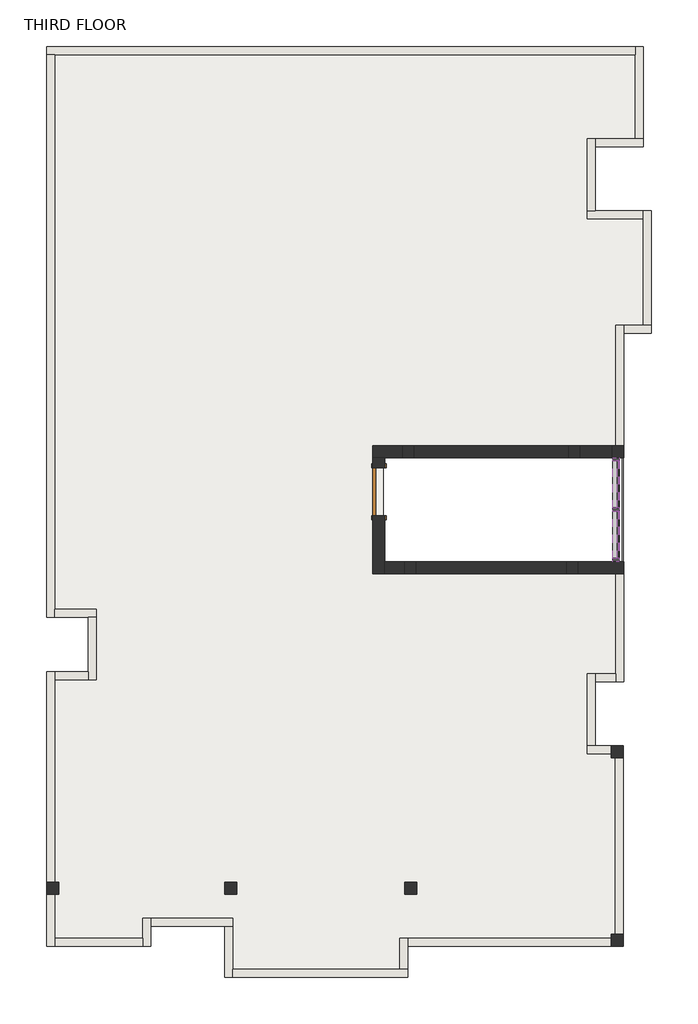
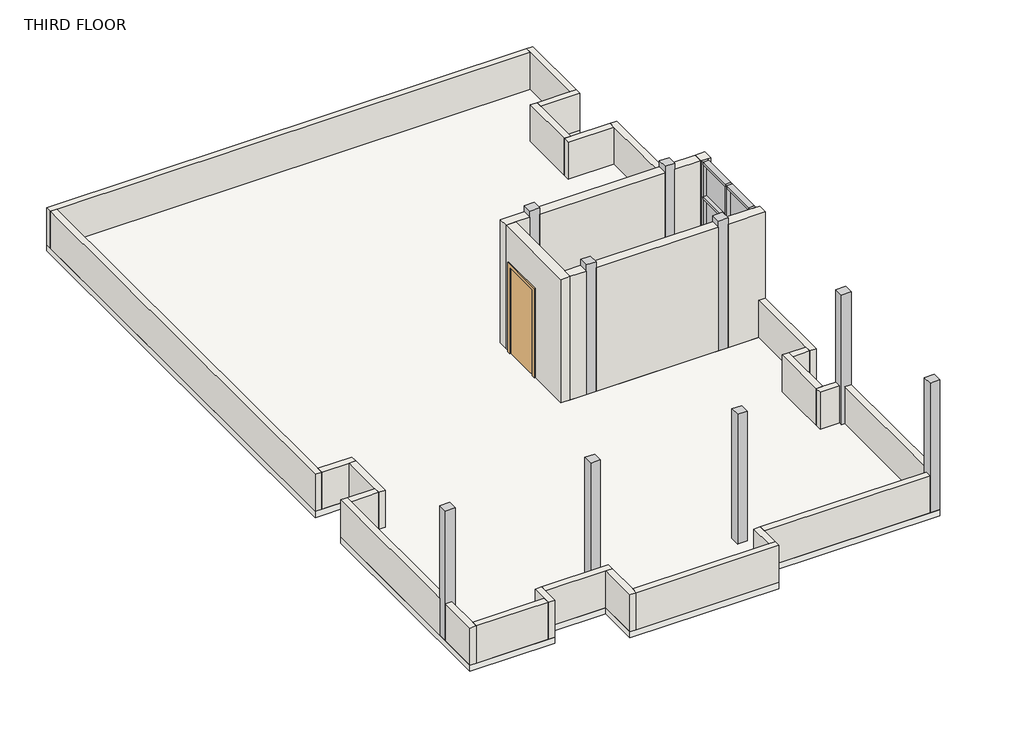
# One storey: 34 walls, 17 members, 9 columns, 6 plates, 1 door, 1 slab.
"""IFC4 building model written with IfcOpenShell, lengths in millimetres."""

from ifc_helpers import new_model, si_unit, frame, origin, place, context, project, spatial, polyline, outline, extrude, faceted_brep, transform, mapped, element, save
from components import single_flush_3_x7_0ca8825f, member_f1f71bde, member_e0487b50, member_e80433b6, member_a715cb85, member_049a2e78, member_69c8e218, member_c4de40ee, member_5cd4c5ac, system_panel_glazed_b791fe2b, system_panel_glazed_d4207c9f

model = new_model("IFC4")

# Units and contexts
model_context = context("Model", 3, world=origin())
ifc_project = project(units=[si_unit("LENGTHUNIT", "METRE", prefix="MILLI")], contexts=[model_context])

# Site, building, storey
site = spatial("IfcSite", under=ifc_project)
building = spatial("IfcBuilding", under=site)
storey = spatial("IfcBuildingStorey", under=building, Name="THIRD FLOOR", Elevation=9601.2)

# Columns
placement = place(None, origin())
element("IfcColumn", 1, ObjectType="Rectangular Column : 9\"X9\"", at=placement, inside=storey, context=model_context, shape_type="Brep", body=[
    faceted_brep([(3352.7127672, -504.2212413, 9601.2), (3352.7127672, -732.8212413, 9601.2), (3124.1127672, -732.8212413, 9601.2), (3124.1127672, -504.2212413, 9601.2), (3352.7127672, -504.2212413, 12801.6), (3352.7127672, -732.8212413, 12801.6), (3352.7127672, -732.8212413, 12649.2), (3352.7127672, -504.2212413, 12649.2), (3124.1127672, -732.8212413, 12801.6), (3124.1127672, -732.8212413, 12649.2), (3124.1127672, -504.2212413, 12801.6), (3124.1127672, -504.2212413, 12649.2)], [[[0, 1, 2, 3]], [[4, 5, 6, 1, 0, 7]], [[5, 8, 9, 2, 1, 6]], [[8, 10, 11, 3, 2, 9]], [[10, 4, 7, 0, 3, 11]], [[4, 10, 8, 5]]]),
])
element("IfcColumn", 2, ObjectType="Rectangular Column : 9\"X9\"", at=placement, inside=storey, context=model_context, shape_type="Brep", body=[
    faceted_brep([(269.7035962, -504.2212413, 9601.2), (269.7035962, -732.8212413, 9601.2), (41.1035962, -732.8212413, 9601.2), (41.1035962, -504.2212413, 9601.2), (269.7035962, -504.2212413, 12801.6), (269.7035962, -732.8212413, 12801.6), (269.7035962, -732.8212413, 12649.2), (269.7035962, -504.2212413, 12649.2), (41.1035962, -732.8212413, 12801.6), (41.1035962, -732.8212413, 12649.2), (41.1035962, -504.2212413, 12801.6), (41.1035962, -504.2212413, 12649.2)], [[[0, 1, 2, 3]], [[4, 5, 6, 1, 0, 7]], [[5, 8, 9, 2, 1, 6]], [[8, 10, 11, 3, 2, 9]], [[10, 4, 7, 0, 3, 11]], [[4, 10, 8, 5]]]),
])
element("IfcColumn", 3, ObjectType="Rectangular Column : 9\"X9\"", at=placement, inside=storey, context=model_context, shape_type="Brep", body=[
    faceted_brep([(229.251657, 1705.5787587, 9601.2), (229.251657, 1476.9787587, 9601.2), (0.651657, 1476.9787587, 9601.2), (0.651657, 1705.5787587, 9601.2), (229.251657, 1705.5787587, 12801.6), (229.251657, 1476.9787587, 12801.6), (229.251657, 1476.9787587, 12649.2), (229.251657, 1705.5787587, 12649.2), (0.651657, 1476.9787587, 12801.6), (0.651657, 1476.9787587, 12649.2), (0.651657, 1705.5787587, 12801.6), (0.651657, 1705.5787587, 12649.2)], [[[0, 1, 2, 3]], [[4, 5, 6, 1, 0, 7]], [[5, 8, 9, 2, 1, 6]], [[8, 10, 11, 3, 2, 9]], [[10, 4, 7, 0, 3, 11]], [[4, 10, 8, 5]]]),
])
element("IfcColumn", 4, ObjectType="Rectangular Column : 9\"X9\"", at=placement, inside=storey, context=model_context, shape_type="Brep", body=[
    faceted_brep([(3385.1070369, 1705.5787587, 9601.2), (3385.1070369, 1476.9787587, 9601.2), (3156.5070369, 1476.9787587, 9601.2), (3156.5070369, 1705.5787587, 9601.2), (3385.1070369, 1705.5787587, 12801.6), (3385.1070369, 1476.9787587, 12801.6), (3385.1070369, 1476.9787587, 12649.2), (3385.1070369, 1705.5787587, 12649.2), (3156.5070369, 1476.9787587, 12801.6), (3156.5070369, 1476.9787587, 12649.2), (3156.5070369, 1705.5787587, 12801.6), (3156.5070369, 1705.5787587, 12649.2)], [[[0, 1, 2, 3]], [[4, 5, 6, 1, 0, 7]], [[5, 8, 9, 2, 1, 6]], [[8, 10, 11, 3, 2, 9]], [[10, 4, 7, 0, 3, 11]], [[4, 10, 8, 5]]]),
])
element("IfcColumn", 5, ObjectType="Rectangular Column : 9\"X9\"", at=placement, inside=storey, context=model_context, shape_type="Brep", body=[
    faceted_brep([(-6539.8865981, -6601.1424416, 9601.2), (-6539.8865981, -6829.7424416, 9601.2), (-6616.0865981, -6829.7424416, 9601.2), (-6768.4865981, -6829.7424416, 9601.2), (-6768.4865981, -6601.1424416, 9601.2), (-6616.0865981, -6601.1424416, 9601.2), (-6539.8865981, -6601.1424416, 12801.6), (-6539.8865981, -6829.7424416, 12801.6), (-6768.4865981, -6829.7424416, 12801.6), (-6768.4865981, -6829.7424416, 10515.6), (-6768.4865981, -6601.1424416, 12801.6), (-6768.4865981, -6601.1424416, 10515.6)], [[[0, 1, 2, 3, 4, 5]], [[6, 7, 1, 0]], [[7, 8, 9, 3, 2, 1]], [[8, 10, 11, 4, 3, 9]], [[10, 6, 0, 5, 4, 11]], [[6, 10, 8, 7]]]),
])
element("IfcColumn", 6, ObjectType="Rectangular Column : 9\"X9\"", at=placement, inside=storey, context=model_context, shape_type="SweptSolid", body=[
    extrude(outline(polyline([(-3148.9865981, -6600.2212413), (-3148.9865981, -6828.8212413), (-3377.5865981, -6828.8212413), (-3377.5865981, -6600.2212413), (-3148.9865981, -6600.2212413)])), frame((0.0, 0.0, 9601.2), z_axis=(0.0, 0.0, 1.0), x_axis=(1.0, 0.0, 0.0)), (0.0, 0.0, 1.0), 3200.4),
])
element("IfcColumn", 7, ObjectType="Rectangular Column : 9\"X9\"", at=placement, inside=storey, context=model_context, shape_type="SweptSolid", body=[
    extrude(outline(polyline([(280.0134019, -6601.1424416), (280.0134019, -6829.7424416), (51.4134019, -6829.7424416), (51.4134019, -6601.1424416), (280.0134019, -6601.1424416)])), frame((0.0, 0.0, 9601.2), z_axis=(0.0, 0.0, 1.0), x_axis=(1.0, 0.0, 0.0)), (0.0, 0.0, 1.0), 3200.4),
])
element("IfcColumn", 8, ObjectType="Rectangular Column : 9\"X9\"", at=placement, inside=storey, context=model_context, shape_type="Brep", body=[
    faceted_brep([(4204.3134019, -7590.8212413, 9601.2), (4204.3134019, -7819.4212413, 9601.2), (3975.7134019, -7819.4212413, 9601.2), (3975.7134019, -7667.0212413, 9601.2), (3975.7134019, -7590.8212413, 9601.2), (4051.9134019, -7590.8212413, 9601.2), (4204.3134019, -7590.8212413, 12801.6), (4204.3134019, -7819.4212413, 12801.6), (4204.3134019, -7590.8212413, 10515.6), (3975.7134019, -7819.4212413, 12801.6), (3975.7134019, -7819.4212413, 10515.6), (3975.7134019, -7590.8212413, 12801.6)], [[[0, 1, 2, 3, 4, 5]], [[6, 7, 1, 0, 8]], [[7, 9, 10, 2, 1]], [[9, 11, 4, 3, 2, 10]], [[11, 6, 8, 0, 5, 4]], [[6, 11, 9, 7]]]),
])
element("IfcColumn", 9, ObjectType="Rectangular Column : 9\"X9\"", at=placement, inside=storey, context=model_context, shape_type="Brep", body=[
    faceted_brep([(4204.3134019, -4009.4212413, 9601.2), (4204.3134019, -4238.0212413, 9601.2), (4051.9134019, -4238.0212413, 9601.2), (3975.7134019, -4238.0212413, 9601.2), (3975.7134019, -4161.8212413, 9601.2), (3975.7134019, -4009.4212413, 9601.2), (4204.3134019, -4009.4212413, 12801.6), (4204.3134019, -4238.0212413, 12801.6), (4204.3134019, -4238.0212413, 10515.6), (3975.7134019, -4238.0212413, 12801.6), (3975.7134019, -4009.4212413, 12801.6), (3975.7134019, -4009.4212413, 10515.6)], [[[0, 1, 2, 3, 4, 5]], [[6, 7, 8, 1, 0]], [[7, 9, 3, 2, 1, 8]], [[9, 10, 11, 5, 4, 3]], [[10, 6, 0, 5, 11]], [[6, 10, 9, 7]]]),
])

# Door
single_flush_3_x7_shape = single_flush_3_x7_0ca8825f(model_context)
element("IfcDoor", 10, ObjectType="Single-Flush : 3'X7'", at=placement, inside=storey, context=model_context, shape_type="MappedRepresentation", body=[
    mapped(single_flush_3_x7_shape, transform((-442.1951421, 829.2787587, 9601.2), x_axis=(0.0, 1.0, 0.0), y_axis=(-1.0, 0.0, 0.0), z_axis=(0.0, 0.0, 1.0))),
])

# Members
member_shape = member_f1f71bde(model_context)
element("IfcMember", 11, ObjectType="Rectangular Mullion : 2.5\" x 5\" rectangular", at=placement, inside=storey, context=model_context, shape_type="MappedRepresentation", body=[
    mapped(member_shape, transform((4070.1027712, -440.7212413, 12649.2), x_axis=(0.0, 0.0, 1.0), y_axis=(-1.0, 0.0, 0.0), z_axis=(0.0, -1.0, 0.0))),
])
element("IfcMember", 12, ObjectType="Rectangular Mullion : 2.5\" x 5\" rectangular", at=placement, inside=storey, context=model_context, shape_type="MappedRepresentation", body=[
    mapped(member_shape, transform((4070.1027712, 518.1287587, 12649.2), x_axis=(0.0, 0.0, 1.0), y_axis=(-1.0, 0.0, 0.0), z_axis=(0.0, -1.0, 0.0))),
])
element("IfcMember", 13, ObjectType="Rectangular Mullion : 2.5\" x 5\" rectangular", at=placement, inside=storey, context=model_context, shape_type="MappedRepresentation", body=[
    mapped(member_shape, transform((4070.1027712, 1413.4787587, 9601.2), x_axis=(0.0, 0.0, -1.0), y_axis=(-1.0, 0.0, 0.0), z_axis=(0.0, 1.0, 0.0))),
])
element("IfcMember", 14, ObjectType="Rectangular Mullion : 2.5\" x 5\" rectangular", at=placement, inside=storey, context=model_context, shape_type="MappedRepresentation", body=[
    mapped(member_shape, transform((4070.1027712, 454.6287587, 9601.2), x_axis=(0.0, 0.0, -1.0), y_axis=(-1.0, 0.0, 0.0), z_axis=(0.0, 1.0, 0.0))),
])
member_2_shape = member_e0487b50(model_context)
element("IfcMember", 15, ObjectType="Rectangular Mullion : 2.5\" x 5\" rectangular", at=placement, inside=storey, context=model_context, shape_type="MappedRepresentation", body=[
    mapped(member_2_shape, transform((4070.1027712, 518.1287587, 10699.75), x_axis=(0.0, 0.0, 1.0), y_axis=(-1.0, 0.0, 0.0), z_axis=(0.0, -1.0, 0.0))),
])
element("IfcMember", 16, ObjectType="Rectangular Mullion : 2.5\" x 5\" rectangular", at=placement, inside=storey, context=model_context, shape_type="MappedRepresentation", body=[
    mapped(member_2_shape, transform((4070.1027712, -440.7212413, 10699.75), x_axis=(0.0, 0.0, 1.0), y_axis=(-1.0, 0.0, 0.0), z_axis=(0.0, -1.0, 0.0))),
])
element("IfcMember", 17, ObjectType="Rectangular Mullion : 2.5\" x 5\" rectangular", at=placement, inside=storey, context=model_context, shape_type="MappedRepresentation", body=[
    mapped(member_2_shape, transform((4070.1027712, 518.1287587, 11766.55), x_axis=(0.0, 0.0, 1.0), y_axis=(-1.0, 0.0, 0.0), z_axis=(0.0, -1.0, 0.0))),
])
element("IfcMember", 18, ObjectType="Rectangular Mullion : 2.5\" x 5\" rectangular", at=placement, inside=storey, context=model_context, shape_type="MappedRepresentation", body=[
    mapped(member_2_shape, transform((4070.1027712, -440.7212413, 11766.55), x_axis=(0.0, 0.0, 1.0), y_axis=(-1.0, 0.0, 0.0), z_axis=(0.0, -1.0, 0.0))),
])
member_3_shape = member_e80433b6(model_context)
element("IfcMember", 19, ObjectType="Rectangular Mullion : 2.5\" x 5\" rectangular", at=placement, inside=storey, context=model_context, shape_type="MappedRepresentation", body=[
    mapped(member_3_shape, transform((4070.1027712, 486.3787587, 9601.2), x_axis=(0.0, -1.0, 0.0), y_axis=(-1.0, 0.0, 0.0), z_axis=(0.0, 0.0, -1.0))),
])
member_4_shape = member_a715cb85(model_context)
element("IfcMember", 20, ObjectType="Rectangular Mullion : 2.5\" x 5\" rectangular", at=placement, inside=storey, context=model_context, shape_type="MappedRepresentation", body=[
    mapped(member_4_shape, transform((4070.1027712, 486.3787587, 10699.75), x_axis=(0.0, -1.0, 0.0), y_axis=(-1.0, 0.0, 0.0), z_axis=(0.0, 0.0, -1.0))),
])
member_5_shape = member_049a2e78(model_context)
element("IfcMember", 21, ObjectType="Rectangular Mullion : 2.5\" x 5\" rectangular", at=placement, inside=storey, context=model_context, shape_type="MappedRepresentation", body=[
    mapped(member_5_shape, transform((4070.1027712, 486.3787587, 11766.55), x_axis=(0.0, -1.0, 0.0), y_axis=(-1.0, 0.0, 0.0), z_axis=(0.0, 0.0, -1.0))),
])
member_6_shape = member_69c8e218(model_context)
element("IfcMember", 22, ObjectType="Rectangular Mullion : 2.5\" x 5\" rectangular", at=placement, inside=storey, context=model_context, shape_type="MappedRepresentation", body=[
    mapped(member_6_shape, transform((4070.1027712, -504.2212413, 9601.2), x_axis=(0.0, -1.0, 0.0), y_axis=(-1.0, 0.0, 0.0), z_axis=(0.0, 0.0, -1.0))),
])
member_7_shape = member_c4de40ee(model_context)
element("IfcMember", 23, ObjectType="Rectangular Mullion : 2.5\" x 5\" rectangular", at=placement, inside=storey, context=model_context, shape_type="MappedRepresentation", body=[
    mapped(member_7_shape, transform((4070.1027712, -504.2212413, 10699.75), x_axis=(0.0, -1.0, 0.0), y_axis=(-1.0, 0.0, 0.0), z_axis=(0.0, 0.0, -1.0))),
])
member_8_shape = member_5cd4c5ac(model_context)
element("IfcMember", 24, ObjectType="Rectangular Mullion : 2.5\" x 5\" rectangular", at=placement, inside=storey, context=model_context, shape_type="MappedRepresentation", body=[
    mapped(member_8_shape, transform((4070.1027712, -504.2212413, 11766.55), x_axis=(0.0, -1.0, 0.0), y_axis=(-1.0, 0.0, 0.0), z_axis=(0.0, 0.0, -1.0))),
])
element("IfcMember", 25, ObjectType="Rectangular Mullion : 2.5\" x 5\" rectangular", at=placement, inside=storey, context=model_context, shape_type="MappedRepresentation", body=[
    mapped(member_8_shape, transform((4070.1027712, 1476.9787587, 12649.2), x_axis=(0.0, 1.0, 0.0), y_axis=(-1.0, 0.0, 0.0), z_axis=(0.0, 0.0, 1.0))),
])
element("IfcMember", 26, ObjectType="Rectangular Mullion : 2.5\" x 5\" rectangular", at=placement, inside=storey, context=model_context, shape_type="MappedRepresentation", body=[
    mapped(member_6_shape, transform((4070.1027712, 1476.9787587, 10699.75), x_axis=(0.0, 1.0, 0.0), y_axis=(-1.0, 0.0, 0.0), z_axis=(0.0, 0.0, 1.0))),
])
element("IfcMember", 27, ObjectType="Rectangular Mullion : 2.5\" x 5\" rectangular", at=placement, inside=storey, context=model_context, shape_type="MappedRepresentation", body=[
    mapped(member_7_shape, transform((4070.1027712, 1476.9787587, 11766.55), x_axis=(0.0, 1.0, 0.0), y_axis=(-1.0, 0.0, 0.0), z_axis=(0.0, 0.0, 1.0))),
])

# Plates
system_panel_glazed_shape = system_panel_glazed_b791fe2b(model_context)
element("IfcPlate", 28, ObjectType="System Panel : Glazed", at=placement, inside=storey, context=model_context, shape_type="MappedRepresentation", body=[
    mapped(system_panel_glazed_shape, transform((4070.1027712, 965.8037587, 9664.7), x_axis=(0.0, -1.0, 0.0), y_axis=(1.0, 0.0, 0.0), z_axis=(0.0, 0.0, 1.0))),
])
element("IfcPlate", 29, ObjectType="System Panel : Glazed", at=placement, inside=storey, context=model_context, shape_type="MappedRepresentation", body=[
    mapped(system_panel_glazed_shape, transform((4070.1027712, 6.9537587, 9664.7), x_axis=(0.0, -1.0, 0.0), y_axis=(1.0, 0.0, 0.0), z_axis=(0.0, 0.0, 1.0))),
])
element("IfcPlate", 30, ObjectType="System Panel : Glazed", at=placement, inside=storey, context=model_context, shape_type="MappedRepresentation", body=[
    mapped(system_panel_glazed_shape, transform((4070.1027712, 965.8037587, 10731.5), x_axis=(0.0, -1.0, 0.0), y_axis=(1.0, 0.0, 0.0), z_axis=(0.0, 0.0, 1.0))),
])
element("IfcPlate", 31, ObjectType="System Panel : Glazed", at=placement, inside=storey, context=model_context, shape_type="MappedRepresentation", body=[
    mapped(system_panel_glazed_shape, transform((4070.1027712, 6.9537587, 10731.5), x_axis=(0.0, -1.0, 0.0), y_axis=(1.0, 0.0, 0.0), z_axis=(0.0, 0.0, 1.0))),
])
system_panel_glazed_2_shape = system_panel_glazed_d4207c9f(model_context)
element("IfcPlate", 32, ObjectType="System Panel : Glazed", at=placement, inside=storey, context=model_context, shape_type="MappedRepresentation", body=[
    mapped(system_panel_glazed_2_shape, transform((4070.1027712, 965.8037587, 11798.3), x_axis=(0.0, -1.0, 0.0), y_axis=(1.0, 0.0, 0.0), z_axis=(0.0, 0.0, 1.0))),
])
element("IfcPlate", 33, ObjectType="System Panel : Glazed", at=placement, inside=storey, context=model_context, shape_type="MappedRepresentation", body=[
    mapped(system_panel_glazed_2_shape, transform((4070.1027712, 6.9537587, 11798.3), x_axis=(0.0, -1.0, 0.0), y_axis=(1.0, 0.0, 0.0), z_axis=(0.0, 0.0, 1.0))),
])

# Slab
element("IfcSlab", 34, ObjectType="6\"", at=placement, inside=storey, context=model_context, shape_type="SweptSolid", body=[
    extrude(outline(polyline([(-6768.4865981, -1558.3212413), (-6768.4865981, 9300.1787587), (4585.3134019, 9300.1787587), (4585.3134019, 7395.1787587), (3670.9134019, 7395.1787587), (3670.9134019, 6175.9787587), (4737.7134019, 6175.9787587), (4737.7134019, 3839.1787587), (4204.3134019, 3839.1787587), (4204.3134019, -2790.2212413), (3670.9134019, -2790.2212413), (3670.9134019, -4009.4212413), (4204.3134019, -4009.4212413), (4204.3134019, -7819.4212413), (102.2134019, -7819.4212413), (102.2134019, -8416.3212413), (-3377.5865981, -8416.3212413), (-3377.5865981, -7438.4212413), (-4787.2865981, -7438.4212413), (-4787.2865981, -7819.4212413), (-6768.4865981, -7819.4212413), (-6768.4865981, -2599.7212413), (-5974.2886947, -2599.7212413), (-5974.2886947, -1558.3212413), (-6768.4865981, -1558.3212413)]), holes=[polyline([(4178.9134019, 1705.5787587), (-353.2951421, 1705.5787587), (-353.2951421, -732.8212413), (4178.9134019, -732.8212413), (4178.9134019, 1705.5787587)])]), frame((0.0, 0.0, 9448.8), z_axis=(0.0, 0.0, 1.0), x_axis=(1.0, 0.0, 0.0)), (0.0, 0.0, 1.0), 152.4),
])

# Walls
element("IfcWall", 35, ObjectType="6\"", at=placement, inside=storey, context=model_context, shape_type="Brep", body=[
    faceted_brep([(-6768.4865981, -2599.7212413, 9601.2), (-6768.4865981, -6601.1424416, 9601.2), (-6768.4865981, -6601.1424416, 10515.6), (-6768.4865981, -2599.7212413, 10515.6), (-6616.0865981, -2599.7212413, 9601.2), (-6616.0865981, -2599.7212413, 10515.6), (-6616.0865981, -2752.1212413, 10515.6), (-6616.0865981, -6601.1424416, 10515.6), (-6616.0865981, -6601.1424416, 9601.2), (-6616.0865981, -2752.1212413, 9601.2)], [[[0, 1, 2, 3]], [[4, 5, 6, 7, 8, 9]], [[1, 0, 4, 9, 8]], [[2, 1, 8, 7]], [[3, 2, 7, 6, 5]], [[0, 3, 5, 4]]]),
])
element("IfcWall", 36, ObjectType="6\"", at=placement, inside=storey, context=model_context, shape_type="Brep", body=[
    faceted_brep([(-6768.4865981, -6829.7424416, 9601.2), (-6768.4865981, -7819.4212413, 9601.2), (-6768.4865981, -7819.4212413, 10515.6), (-6768.4865981, -6829.7424416, 10515.6), (-6616.0865981, -6829.7424416, 9601.2), (-6616.0865981, -6829.7424416, 10515.6), (-6616.0865981, -7667.0212413, 10515.6), (-6616.0865981, -7819.4212413, 10515.6), (-6616.0865981, -7819.4212413, 9601.2), (-6616.0865981, -7667.0212413, 9601.2)], [[[0, 1, 2, 3]], [[4, 5, 6, 7, 8, 9]], [[1, 0, 4, 9, 8]], [[3, 2, 7, 6, 5]], [[0, 3, 5, 4]], [[2, 1, 8, 7]]]),
])
element("IfcWall", 37, ObjectType="6\"", at=placement, inside=storey, context=model_context, shape_type="SweptSolid", body=[
    extrude(outline(polyline([(-4939.6865981, -7819.4212413), (-6616.0865981, -7819.4212413), (-6616.0865981, -7667.0212413), (-4939.6865981, -7667.0212413), (-4939.6865981, -7819.4212413)])), frame((0.0, 0.0, 9601.2), z_axis=(0.0, 0.0, 1.0), x_axis=(1.0, 0.0, 0.0)), (0.0, 0.0, 1.0), 914.4),
])
element("IfcWall", 38, ObjectType="6\"", at=placement, inside=storey, context=model_context, shape_type="Brep", body=[
    faceted_brep([(-4787.2865981, -7819.4212413, 9601.2), (-4787.2865981, -7438.4212413, 9601.2), (-4787.2865981, -7286.0212413, 9601.2), (-4787.2865981, -7286.0212413, 10515.6), (-4787.2865981, -7438.4212413, 10515.6), (-4787.2865981, -7819.4212413, 10515.6), (-4939.6865981, -7819.4212413, 9601.2), (-4939.6865981, -7819.4212413, 10515.6), (-4939.6865981, -7667.0212413, 10515.6), (-4939.6865981, -7286.0212413, 10515.6), (-4939.6865981, -7286.0212413, 9601.2), (-4939.6865981, -7667.0212413, 9601.2)], [[[0, 1, 2, 3, 4, 5]], [[6, 7, 8, 9, 10, 11]], [[2, 1, 0, 6, 11, 10]], [[5, 4, 3, 9, 8, 7]], [[0, 5, 7, 6]], [[3, 2, 10, 9]]]),
])
element("IfcWall", 39, ObjectType="6\"", at=placement, inside=storey, context=model_context, shape_type="Brep", body=[
    faceted_brep([(-4787.2865981, -7438.4212413, 9601.2), (-3377.5865981, -7438.4212413, 9601.2), (-3225.1865981, -7438.4212413, 9601.2), (-3225.1865981, -7438.4212413, 10515.6), (-3377.5865981, -7438.4212413, 10515.6), (-4787.2865981, -7438.4212413, 10515.6), (-4787.2865981, -7286.0212413, 9601.2), (-4787.2865981, -7286.0212413, 10515.6), (-3225.1865981, -7286.0212413, 10515.6), (-3225.1865981, -7286.0212413, 9601.2)], [[[0, 1, 2, 3, 4, 5]], [[6, 7, 8, 9]], [[2, 1, 0, 6, 9]], [[5, 4, 3, 8, 7]], [[0, 5, 7, 6]], [[3, 2, 9, 8]]]),
])
element("IfcWall", 40, ObjectType="6\"", at=placement, inside=storey, context=model_context, shape_type="Brep", body=[
    faceted_brep([(-3377.5865981, -7438.4212413, 9601.2), (-3377.5865981, -8416.3212413, 9601.2), (-3377.5865981, -8416.3212413, 10515.6), (-3377.5865981, -7438.4212413, 10515.6), (-3225.1865981, -7438.4212413, 9601.2), (-3225.1865981, -7438.4212413, 10515.6), (-3225.1865981, -8263.9212413, 10515.6), (-3225.1865981, -8416.3212413, 10515.6), (-3225.1865981, -8416.3212413, 9601.2), (-3225.1865981, -8263.9212413, 9601.2)], [[[0, 1, 2, 3]], [[4, 5, 6, 7, 8, 9]], [[1, 0, 4, 9, 8]], [[3, 2, 7, 6, 5]], [[0, 3, 5, 4]], [[2, 1, 8, 7]]]),
])
element("IfcWall", 41, ObjectType="6\"", at=placement, inside=storey, context=model_context, shape_type="Brep", body=[
    faceted_brep([(-3225.1865981, -8416.3212413, 9601.2), (102.2134019, -8416.3212413, 9601.2), (102.2134019, -8416.3212413, 10515.6), (-3225.1865981, -8416.3212413, 10515.6), (-3225.1865981, -8263.9212413, 9601.2), (-3225.1865981, -8263.9212413, 10515.6), (-50.1865981, -8263.9212413, 10515.6), (102.2134019, -8263.9212413, 10515.6), (102.2134019, -8263.9212413, 9601.2), (-50.1865981, -8263.9212413, 9601.2)], [[[0, 1, 2, 3]], [[4, 5, 6, 7, 8, 9]], [[1, 0, 4, 9, 8]], [[3, 2, 7, 6, 5]], [[0, 3, 5, 4]], [[2, 1, 8, 7]]]),
])
element("IfcWall", 42, ObjectType="6\"", at=placement, inside=storey, context=model_context, shape_type="Brep", body=[
    faceted_brep([(102.2134019, -8263.9212413, 9601.2), (102.2134019, -7819.4212413, 9601.2), (102.2134019, -7667.0212413, 9601.2), (102.2134019, -7667.0212413, 10515.6), (102.2134019, -7819.4212413, 10515.6), (102.2134019, -8263.9212413, 10515.6), (-50.1865981, -8263.9212413, 9601.2), (-50.1865981, -8263.9212413, 10515.6), (-50.1865981, -7667.0212413, 10515.6), (-50.1865981, -7667.0212413, 9601.2)], [[[0, 1, 2, 3, 4, 5]], [[6, 7, 8, 9]], [[2, 1, 0, 6, 9]], [[5, 4, 3, 8, 7]], [[0, 5, 7, 6]], [[3, 2, 9, 8]]]),
])
element("IfcWall", 43, ObjectType="6\"", at=placement, inside=storey, context=model_context, shape_type="SweptSolid", body=[
    extrude(outline(polyline([(3975.7134019, -7819.4212413), (102.2134019, -7819.4212413), (102.2134019, -7667.0212413), (3975.7134019, -7667.0212413), (3975.7134019, -7819.4212413)])), frame((0.0, 0.0, 9601.2), z_axis=(0.0, 0.0, 1.0), x_axis=(1.0, 0.0, 0.0)), (0.0, 0.0, 1.0), 914.4),
])
element("IfcWall", 44, ObjectType="6\"", at=placement, inside=storey, context=model_context, shape_type="SweptSolid", body=[
    extrude(outline(polyline([(4204.3134019, -4238.0212413), (4204.3134019, -7590.8212413), (4051.9134019, -7590.8212413), (4051.9134019, -4238.0212413), (4204.3134019, -4238.0212413)])), frame((0.0, 0.0, 9601.2), z_axis=(0.0, 0.0, 1.0), x_axis=(1.0, 0.0, 0.0)), (0.0, 0.0, 1.0), 914.4),
])
element("IfcWall", 45, ObjectType="6\"", at=placement, inside=storey, context=model_context, shape_type="Brep", body=[
    faceted_brep([(3975.7134019, -4009.4212413, 9601.2), (3670.9134019, -4009.4212413, 9601.2), (3518.5134019, -4009.4212413, 9601.2), (3518.5134019, -4009.4212413, 10515.6), (3670.9134019, -4009.4212413, 10515.6), (3975.7134019, -4009.4212413, 10515.6), (3975.7134019, -4161.8212413, 9601.2), (3975.7134019, -4161.8212413, 10515.6), (3518.5134019, -4161.8212413, 10515.6), (3518.5134019, -4161.8212413, 9601.2)], [[[0, 1, 2, 3, 4, 5]], [[6, 7, 8, 9]], [[2, 1, 0, 6, 9]], [[5, 4, 3, 8, 7]], [[0, 5, 7, 6]], [[3, 2, 9, 8]]]),
])
element("IfcWall", 46, ObjectType="6\"", at=placement, inside=storey, context=model_context, shape_type="Brep", body=[
    faceted_brep([(3670.9134019, -4009.4212413, 9601.2), (3670.9134019, -2790.2212413, 9601.2), (3670.9134019, -2637.8212413, 9601.2), (3670.9134019, -2637.8212413, 10515.6), (3670.9134019, -2790.2212413, 10515.6), (3670.9134019, -4009.4212413, 10515.6), (3518.5134019, -4009.4212413, 9601.2), (3518.5134019, -4009.4212413, 10515.6), (3518.5134019, -2637.8212413, 10515.6), (3518.5134019, -2637.8212413, 9601.2)], [[[0, 1, 2, 3, 4, 5]], [[6, 7, 8, 9]], [[2, 1, 0, 6, 9]], [[5, 4, 3, 8, 7]], [[0, 5, 7, 6]], [[3, 2, 9, 8]]]),
])
element("IfcWall", 47, ObjectType="6\"", at=placement, inside=storey, context=model_context, shape_type="SweptSolid", body=[
    extrude(outline(polyline([(4064.6134019, -2790.2212413), (3670.9134019, -2790.2212413), (3670.9134019, -2637.8212413), (4064.6134019, -2637.8212413), (4064.6134019, -2790.2212413)])), frame((0.0, 0.0, 9601.2), z_axis=(0.0, 0.0, 1.0), x_axis=(1.0, 0.0, 0.0)), (0.0, 0.0, 1.0), 914.4),
])
element("IfcWall", 48, ObjectType="6\"", at=placement, inside=storey, context=model_context, shape_type="Brep", body=[
    faceted_brep([(4217.0134019, -2790.2212413, 9601.2), (4217.0134019, -732.8212413, 9601.2), (4217.0134019, -732.8212413, 10515.6), (4217.0134019, -2790.2212413, 10515.6), (4064.6134019, -2790.2212413, 9601.2), (4064.6134019, -2790.2212413, 10515.6), (4064.6134019, -2637.8212413, 10515.6), (4064.6134019, -732.8212413, 10515.6), (4064.6134019, -732.8212413, 9601.2), (4064.6134019, -2637.8212413, 9601.2)], [[[0, 1, 2, 3]], [[4, 5, 6, 7, 8, 9]], [[1, 0, 4, 9, 8]], [[3, 2, 7, 6, 5]], [[2, 1, 8, 7]], [[0, 3, 5, 4]]]),
])
element("IfcWall", 49, ObjectType="6\"", at=placement, inside=storey, context=model_context, shape_type="Brep", body=[
    faceted_brep([(4217.0134019, 1705.5787587, 9601.2), (4217.0134019, 3839.1787587, 9601.2), (4217.0134019, 3991.5787587, 9601.2), (4217.0134019, 3991.5787587, 10515.6), (4217.0134019, 3839.1787587, 10515.6), (4217.0134019, 1705.5787587, 10515.6), (4064.6134019, 1705.5787587, 9601.2), (4064.6134019, 1705.5787587, 10515.6), (4064.6134019, 3991.5787587, 10515.6), (4064.6134019, 3991.5787587, 9601.2)], [[[0, 1, 2, 3, 4, 5]], [[6, 7, 8, 9]], [[2, 1, 0, 6, 9]], [[5, 4, 3, 8, 7]], [[0, 5, 7, 6]], [[3, 2, 9, 8]]]),
])
element("IfcWall", 50, ObjectType="6\"", at=placement, inside=storey, context=model_context, shape_type="Brep", body=[
    faceted_brep([(4217.0134019, 3839.1787587, 9601.2), (4737.7134019, 3839.1787587, 9601.2), (4737.7134019, 3839.1787587, 10515.6), (4217.0134019, 3839.1787587, 10515.6), (4217.0134019, 3991.5787587, 9601.2), (4217.0134019, 3991.5787587, 10515.6), (4585.3134019, 3991.5787587, 10515.6), (4737.7134019, 3991.5787587, 10515.6), (4737.7134019, 3991.5787587, 9601.2), (4585.3134019, 3991.5787587, 9601.2)], [[[0, 1, 2, 3]], [[4, 5, 6, 7, 8, 9]], [[1, 0, 4, 9, 8]], [[3, 2, 7, 6, 5]], [[0, 3, 5, 4]], [[2, 1, 8, 7]]]),
])
element("IfcWall", 51, ObjectType="6\"", at=placement, inside=storey, context=model_context, shape_type="Brep", body=[
    faceted_brep([(4737.7134019, 3991.5787587, 9601.2), (4737.7134019, 6175.9787587, 9601.2), (4737.7134019, 6175.9787587, 10515.6), (4737.7134019, 3991.5787587, 10515.6), (4585.3134019, 3991.5787587, 9601.2), (4585.3134019, 3991.5787587, 10515.6), (4585.3134019, 6023.5787587, 10515.6), (4585.3134019, 6175.9787587, 10515.6), (4585.3134019, 6175.9787587, 9601.2), (4585.3134019, 6023.5787587, 9601.2)], [[[0, 1, 2, 3]], [[4, 5, 6, 7, 8, 9]], [[1, 0, 4, 9, 8]], [[3, 2, 7, 6, 5]], [[0, 3, 5, 4]], [[2, 1, 8, 7]]]),
])
element("IfcWall", 52, ObjectType="6\"", at=placement, inside=storey, context=model_context, shape_type="Brep", body=[
    faceted_brep([(4585.3134019, 6175.9787587, 9601.2), (3670.9134019, 6175.9787587, 9601.2), (3518.5134019, 6175.9787587, 9601.2), (3518.5134019, 6175.9787587, 10515.6), (3670.9134019, 6175.9787587, 10515.6), (4585.3134019, 6175.9787587, 10515.6), (4585.3134019, 6023.5787587, 9601.2), (4585.3134019, 6023.5787587, 10515.6), (3518.5134019, 6023.5787587, 10515.6), (3518.5134019, 6023.5787587, 9601.2)], [[[0, 1, 2, 3, 4, 5]], [[6, 7, 8, 9]], [[2, 1, 0, 6, 9]], [[5, 4, 3, 8, 7]], [[0, 5, 7, 6]], [[3, 2, 9, 8]]]),
])
element("IfcWall", 53, ObjectType="6\"", at=placement, inside=storey, context=model_context, shape_type="Brep", body=[
    faceted_brep([(3670.9134019, 6175.9787587, 9601.2), (3670.9134019, 7395.1787587, 9601.2), (3670.9134019, 7547.5787587, 9601.2), (3670.9134019, 7547.5787587, 10515.6), (3670.9134019, 7395.1787587, 10515.6), (3670.9134019, 6175.9787587, 10515.6), (3518.5134019, 6175.9787587, 9601.2), (3518.5134019, 6175.9787587, 10515.6), (3518.5134019, 7547.5787587, 10515.6), (3518.5134019, 7547.5787587, 9601.2)], [[[0, 1, 2, 3, 4, 5]], [[6, 7, 8, 9]], [[2, 1, 0, 6, 9]], [[5, 4, 3, 8, 7]], [[0, 5, 7, 6]], [[3, 2, 9, 8]]]),
])
element("IfcWall", 54, ObjectType="6\"", at=placement, inside=storey, context=model_context, shape_type="Brep", body=[
    faceted_brep([(3670.9134019, 7395.1787587, 9601.2), (4585.3134019, 7395.1787587, 9601.2), (4585.3134019, 7395.1787587, 10515.6), (3670.9134019, 7395.1787587, 10515.6), (3670.9134019, 7547.5787587, 9601.2), (3670.9134019, 7547.5787587, 10515.6), (4432.9134019, 7547.5787587, 10515.6), (4585.3134019, 7547.5787587, 10515.6), (4585.3134019, 7547.5787587, 9601.2), (4432.9134019, 7547.5787587, 9601.2)], [[[0, 1, 2, 3]], [[4, 5, 6, 7, 8, 9]], [[1, 0, 4, 9, 8]], [[3, 2, 7, 6, 5]], [[0, 3, 5, 4]], [[2, 1, 8, 7]]]),
])
element("IfcWall", 55, ObjectType="6\"", at=placement, inside=storey, context=model_context, shape_type="Brep", body=[
    faceted_brep([(4585.3134019, 7547.5787587, 9601.2), (4585.3134019, 9300.1787587, 9601.2), (4585.3134019, 9300.1787587, 10515.6), (4585.3134019, 7547.5787587, 10515.6), (4432.9134019, 7547.5787587, 9601.2), (4432.9134019, 7547.5787587, 10515.6), (4432.9134019, 9147.7787587, 10515.6), (4432.9134019, 9300.1787587, 10515.6), (4432.9134019, 9300.1787587, 9601.2), (4432.9134019, 9147.7787587, 9601.2)], [[[0, 1, 2, 3]], [[4, 5, 6, 7, 8, 9]], [[1, 0, 4, 9, 8]], [[3, 2, 7, 6, 5]], [[0, 3, 5, 4]], [[2, 1, 8, 7]]]),
])
element("IfcWall", 56, ObjectType="6\"", at=placement, inside=storey, context=model_context, shape_type="Brep", body=[
    faceted_brep([(4432.9134019, 9300.1787587, 9601.2), (-6768.4865981, 9300.1787587, 9601.2), (-6768.4865981, 9300.1787587, 10515.6), (4432.9134019, 9300.1787587, 10515.6), (4432.9134019, 9147.7787587, 9601.2), (4432.9134019, 9147.7787587, 10515.6), (-6616.0865981, 9147.7787587, 10515.6), (-6768.4865981, 9147.7787587, 10515.6), (-6768.4865981, 9147.7787587, 9601.2), (-6616.0865981, 9147.7787587, 9601.2)], [[[0, 1, 2, 3]], [[4, 5, 6, 7, 8, 9]], [[1, 0, 4, 9, 8]], [[3, 2, 7, 6, 5]], [[0, 3, 5, 4]], [[2, 1, 8, 7]]]),
])
element("IfcWall", 57, ObjectType="6\"", at=placement, inside=storey, context=model_context, shape_type="Brep", body=[
    faceted_brep([(-6768.4865981, 9147.7787587, 9601.2), (-6768.4865981, -1558.3212413, 9601.2), (-6768.4865981, -1558.3212413, 10515.6), (-6768.4865981, 9147.7787587, 10515.6), (-6616.0865981, 9147.7787587, 9601.2), (-6616.0865981, 9147.7787587, 10515.6), (-6616.0865981, -1405.9212413, 10515.6), (-6616.0865981, -1558.3212413, 10515.6), (-6616.0865981, -1558.3212413, 9601.2), (-6616.0865981, -1405.9212413, 9601.2)], [[[0, 1, 2, 3]], [[4, 5, 6, 7, 8, 9]], [[1, 0, 4, 9, 8]], [[3, 2, 7, 6, 5]], [[0, 3, 5, 4]], [[2, 1, 8, 7]]]),
])
element("IfcWall", 58, ObjectType="6\"", at=placement, inside=storey, context=model_context, shape_type="Brep", body=[
    faceted_brep([(-6616.0865981, -1558.3212413, 9601.2), (-5974.2886947, -1558.3212413, 9601.2), (-5821.8886947, -1558.3212413, 9601.2), (-5821.8886947, -1558.3212413, 10515.6), (-5974.2886947, -1558.3212413, 10515.6), (-6616.0865981, -1558.3212413, 10515.6), (-6616.0865981, -1405.9212413, 9601.2), (-6616.0865981, -1405.9212413, 10515.6), (-5821.8886947, -1405.9212413, 10515.6), (-5821.8886947, -1405.9212413, 9601.2)], [[[0, 1, 2, 3, 4, 5]], [[6, 7, 8, 9]], [[2, 1, 0, 6, 9]], [[5, 4, 3, 8, 7]], [[3, 2, 9, 8]], [[0, 5, 7, 6]]]),
])
element("IfcWall", 59, ObjectType="6\"", at=placement, inside=storey, context=model_context, shape_type="Brep", body=[
    faceted_brep([(-5974.2886947, -1558.3212413, 9601.2), (-5974.2886947, -2599.7212413, 9601.2), (-5974.2886947, -2752.1212413, 9601.2), (-5974.2886947, -2752.1212413, 10515.6), (-5974.2886947, -2599.7212413, 10515.6), (-5974.2886947, -1558.3212413, 10515.6), (-5821.8886947, -1558.3212413, 9601.2), (-5821.8886947, -1558.3212413, 10515.6), (-5821.8886947, -2752.1212413, 10515.6), (-5821.8886947, -2752.1212413, 9601.2)], [[[0, 1, 2, 3, 4, 5]], [[6, 7, 8, 9]], [[2, 1, 0, 6, 9]], [[5, 4, 3, 8, 7]], [[0, 5, 7, 6]], [[3, 2, 9, 8]]]),
])
element("IfcWall", 60, ObjectType="6\"", at=placement, inside=storey, context=model_context, shape_type="SweptSolid", body=[
    extrude(outline(polyline([(-6616.0865981, -2599.7212413), (-5974.2886947, -2599.7212413), (-5974.2886947, -2752.1212413), (-6616.0865981, -2752.1212413), (-6616.0865981, -2599.7212413)])), frame((0.0, 0.0, 9601.2), z_axis=(0.0, 0.0, 1.0), x_axis=(1.0, 0.0, 0.0)), (0.0, 0.0, 1.0), 914.4),
])
element("IfcWall", 61, ObjectType="9\"", at=placement, inside=storey, context=model_context, shape_type="SweptSolid", body=[
    extrude(outline(polyline([(3124.1127672, -732.8212413), (269.7035962, -732.8212413), (269.7035962, -504.2212413), (3124.1127672, -504.2212413), (3124.1127672, -732.8212413)])), frame((0.0, 0.0, 9601.2), z_axis=(0.0, 0.0, 1.0), x_axis=(1.0, 0.0, 0.0)), (0.0, 0.0, 1.0), 3048.0),
])
element("IfcWall", 62, ObjectType="9\"", at=placement, inside=storey, context=model_context, shape_type="Brep", body=[
    faceted_brep([(3352.7127672, -732.8212413, 9601.2), (4064.6134019, -732.8212413, 9601.2), (4217.0134019, -732.8212413, 9601.2), (4217.0134019, -732.8212413, 10515.6), (4217.0134019, -732.8212413, 12649.2), (3352.7127672, -732.8212413, 12649.2), (3352.7127672, -504.2212413, 9601.2), (3352.7127672, -504.2212413, 12649.2), (3988.4134019, -504.2212413, 12649.2), (4217.0134019, -504.2212413, 12649.2), (4217.0134019, -504.2212413, 9601.2), (3988.4134019, -504.2212413, 9601.2)], [[[0, 1, 2, 3, 4, 5]], [[6, 7, 8, 9, 10, 11]], [[2, 1, 0, 6, 11, 10]], [[5, 4, 9, 8, 7]], [[0, 5, 7, 6]], [[2, 10, 9, 4, 3]]]),
])
element("IfcWall", 63, ObjectType="9\"", at=placement, inside=storey, context=model_context, shape_type="Brep", body=[
    faceted_brep([(4217.0134019, 1705.5787587, 9601.2), (4217.0134019, 1705.5787587, 10515.6), (4217.0134019, 1705.5787587, 12649.2), (4217.0134019, 1476.9787587, 12649.2), (4217.0134019, 1476.9787587, 9601.2), (3988.4134019, 1705.5787587, 12649.2), (3988.4134019, 1705.5787587, 9601.2), (3988.4134019, 1476.9787587, 9601.2), (3988.4134019, 1476.9787587, 12649.2), (4064.6134019, 1705.5787587, 9601.2)], [[[0, 1, 2, 3, 4]], [[5, 6, 7, 8]], [[6, 9, 0, 4, 7]], [[2, 5, 8, 3]], [[0, 9, 6, 5, 2, 1]], [[4, 3, 8, 7]]]),
])
element("IfcWall", 64, ObjectType="9\"", at=placement, inside=storey, context=model_context, shape_type="SweptSolid", body=[
    extrude(outline(polyline([(3385.1070369, 1705.5787587), (3988.4134019, 1705.5787587), (3988.4134019, 1476.9787587), (3385.1070369, 1476.9787587), (3385.1070369, 1705.5787587)])), frame((0.0, 0.0, 9601.2), z_axis=(0.0, 0.0, 1.0), x_axis=(1.0, 0.0, 0.0)), (0.0, 0.0, 1.0), 3048.0),
])
element("IfcWall", 65, ObjectType="9\"", at=placement, inside=storey, context=model_context, shape_type="SweptSolid", body=[
    extrude(outline(polyline([(229.251657, 1705.5787587), (3156.5070369, 1705.5787587), (3156.5070369, 1476.9787587), (229.251657, 1476.9787587), (229.251657, 1705.5787587)])), frame((0.0, 0.0, 9601.2), z_axis=(0.0, 0.0, 1.0), x_axis=(1.0, 0.0, 0.0)), (0.0, 0.0, 1.0), 3048.0),
])
element("IfcWall", 66, ObjectType="9\"", at=placement, inside=storey, context=model_context, shape_type="Brep", body=[
    faceted_brep([(0.651657, 1705.5787587, 9601.2), (-556.4951421, 1705.5787587, 9601.2), (-556.4951421, 1705.5787587, 12649.2), (0.651657, 1705.5787587, 12649.2), (0.651657, 1476.9787587, 9601.2), (0.651657, 1476.9787587, 12649.2), (-327.8951421, 1476.9787587, 12649.2), (-556.4951421, 1476.9787587, 12649.2), (-556.4951421, 1476.9787587, 9601.2), (-327.8951421, 1476.9787587, 9601.2)], [[[0, 1, 2, 3]], [[4, 5, 6, 7, 8, 9]], [[1, 0, 4, 9, 8]], [[3, 2, 7, 6, 5]], [[0, 3, 5, 4]], [[2, 1, 8, 7]]]),
])
element("IfcWall", 67, ObjectType="9\"", at=placement, inside=storey, context=model_context, shape_type="Brep", body=[
    faceted_brep([(-556.4951421, 1476.9787587, 9601.2), (-556.4951421, 1286.4787587, 9601.2), (-556.4951421, 1286.4787587, 11734.8), (-556.4951421, 372.0787587, 11734.8), (-556.4951421, 372.0787587, 9601.2), (-556.4951421, -732.8212413, 9601.2), (-556.4951421, -732.8212413, 12649.2), (-556.4951421, 1476.9787587, 12649.2), (-327.8951421, 1286.4787587, 11734.8), (-327.8951421, 1286.4787587, 9601.2), (-327.8951421, 1476.9787587, 9601.2), (-327.8951421, 1476.9787587, 12649.2), (-327.8951421, -504.2212413, 12649.2), (-327.8951421, -732.8212413, 12649.2), (-327.8951421, -732.8212413, 9601.2), (-327.8951421, -504.2212413, 9601.2), (-327.8951421, 372.0787587, 9601.2), (-327.8951421, 372.0787587, 11734.8)], [[[0, 1, 2, 3, 4, 5, 6, 7]], [[8, 9, 10, 11, 12, 13, 14, 15, 16, 17]], [[10, 9, 1, 0]], [[16, 15, 14, 5, 4]], [[7, 6, 13, 12, 11]], [[0, 7, 11, 10]], [[6, 5, 14, 13]], [[2, 1, 9, 8]], [[3, 2, 8, 17]], [[4, 3, 17, 16]]]),
])
element("IfcWall", 68, ObjectType="9\"", at=placement, inside=storey, context=model_context, shape_type="SweptSolid", body=[
    extrude(outline(polyline([(41.1035962, -732.8212413), (-327.8951421, -732.8212413), (-327.8951421, -504.2212413), (41.1035962, -504.2212413), (41.1035962, -732.8212413)])), frame((0.0, 0.0, 9601.2), z_axis=(0.0, 0.0, 1.0), x_axis=(1.0, 0.0, 0.0)), (0.0, 0.0, 1.0), 3048.0),
])

save(model, "model.ifc")

# Revit data of these elements
# Type "Rectangular Column : 9\"X9\""
#   Assembly Code = "B1010200"
#   Depth = 0' - 9"
#   Offset Base = 0' - 0"
#   Offset Top = 0' - 0"
#   Width = 0' - 9"
#   Material = none
# Type "Single-Flush : 3'X7'"
#   Type Mark = "8"
#   Construction Type Id = "MDOOR"
#   Assembly Code = "C1020"
#   Analytic Construction = "Metal"
#   Thickness = 0' - 2"
#   Heat Transfer Coefficient (U) = 0.651978 BTU/(h·ft²·°F)
#   Height = 7' - 0"
#   Trim Projection Ext = 0' - 1"
#   Trim Projection Int = 0' - 1"
#   Trim Width = 0' - 3"
#   Width = 3' - 0"
#   Define Thermal Properties by = 1
#   Door Material = Door - Panel
#   Frame Material = Door - Frame
#   Visual Light Transmittance = 0
#   Solar Heat Gain Coefficient = 0
#   Function = (empty or 0)
#   Wall Closure = (empty or 0)
# Type "Rectangular Mullion : 2.5\" x 5\" rectangular"
#   built-in parameter 1007304 = 0.416667 (stored number, unit not read)
#   built-in parameter 1007301 = 0.104167 (stored number, unit not read)
#   built-in parameter 1007300 = 0.104167 (stored number, unit not read)
# Type "System Panel : Glazed"
#   Construction Type Id = "GSP4R"
#   Analytic Construction = "1/8 in Pilkington single glazing"
#   Visual Light Transmittance = 0.9
#   Solar Heat Gain Coefficient = 0.86
#   Heat Transfer Coefficient (U) = 1.18115 BTU/(h·ft²·°F)
#   Define Thermal Properties by = 1
# Type "6\""
#   Assembly Code = "B1010"
#   Function = 0
#   Layers, outside or top first: 0' - 6" no material (function 1)
# Type "6\""
#   Assembly Code = "B2010"
#   Layers, outside or top first: 0' - 6" "wood 1" (function 1)
# Type "9\""
#   Assembly Code = "B2010"
#   Layers, outside or top first: 0' - 9" "wall" (function 1)
# Elements 1, 2, 3, 4 (IfcColumn, "Rectangular Column : 9\"X9\"")
#   Phase Created = New Construction
#   Materials on its faces: "wall"
# Elements 5, 8, 9 (IfcColumn, "Rectangular Column : 9\"X9\"")
#   Phase Created = New Construction
#   Materials on its faces: "wood 1"
# Elements 6, 7 (IfcColumn, "Rectangular Column : 9\"X9\"")
#   Phase Created = New Construction
# Element 10 (IfcDoor, "Single-Flush : 3'X7'")
#   Phase Created = New Construction
#   Materials on its faces: "Door - Frame", "Door - Panel"
# Elements 11, 12, 13, 14, 15, 16, 17, 18, 19, 20, 21, 22, 23, 24, 25, 26, 27 (IfcMember, "Rectangular Mullion : 2.5\" x 5\" rectangular")
#   Phase Created = New Construction
#   Materials on its faces: "Aluminum"
# Elements 28, 29, 30, 31, 32, 33 (IfcPlate, "System Panel : Glazed")
#   Phase Created = New Construction
#   Materials on its faces: "Glass"
# Element 34 (IfcSlab, "6\"")
#   built-in parameter 1001955 = -1.5708 (stored number, unit not read)
#   Height Offset From Level = 0' - 0"
#   Phase Created = New Construction
#   Materials on its faces: "Default Floor", "6\" wall"
# Elements 35, 36, 37, 38, 39, 40, 41, 42, 43, 44, 45, 46, 47, 48, 49, 50, 51, 52, 53, 54, 55, 56, 57, 58, 59, 60 (IfcWall, "6\"")
#   Top Offset = -0' - 6"
#   Base Offset = 0' - 0"
#   Unconnected Height = 3' - 0"
#   wall height = 3' - 0"
#   Phase Created = New Construction
#   Base Constraint = THIRD FLOOR
#   Materials on its faces: "wood 1"
# Elements 61, 62, 63, 64, 65, 66, 67, 68 (IfcWall, "9\"")
#   Top Offset = -0' - 6"
#   Base Offset = 0' - 0"
#   wall height = 10' - 0"
#   Phase Created = New Construction
#   Base Constraint = THIRD FLOOR
#   Top Constraint = ROOF
#   Materials on its faces: "wall"
# Materials
#   "Door - Panel": class "Wood", colour RGB 210 159 95, transparency 0, Cost = 0
#   "Door - Frame": colour RGB 118 70 51, transparency 0, Cost = 0
#   "wood 1": class "Generic", colour RGB 88 94 108, transparency 0, Cost = 0
#   "wall": class "Generic", colour RGB 112 128 144, transparency 0, Cost = 0
#   "Aluminum": class "Metal", colour RGB 247 247 247, transparency 0, Description = "Aluminum 6061", Cost = 0
#   "Glass": class "Glass", colour RGB 0 128 192, transparency 0.75, Description = "Soda Lime Glass", Cost = 0
#   "Default Floor": colour RGB 128 128 128, transparency 0, Cost = 0
#   "6\" wall": class "Generic", colour RGB 250 243 224, transparency 0, Cost = 0
